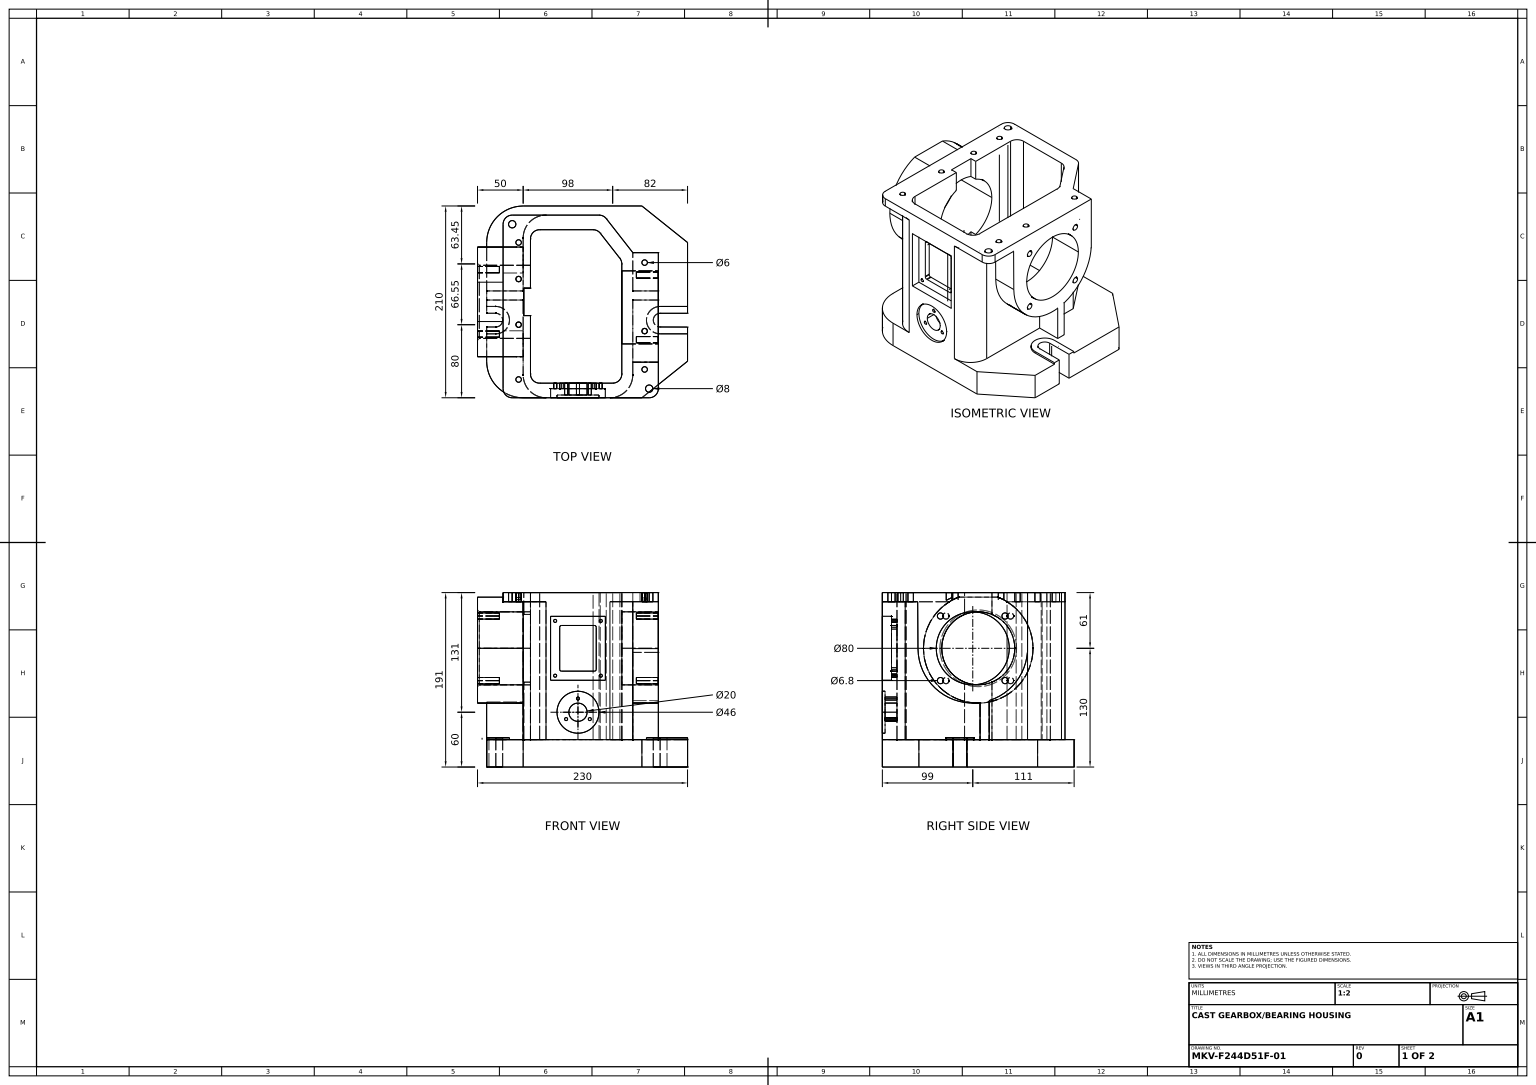
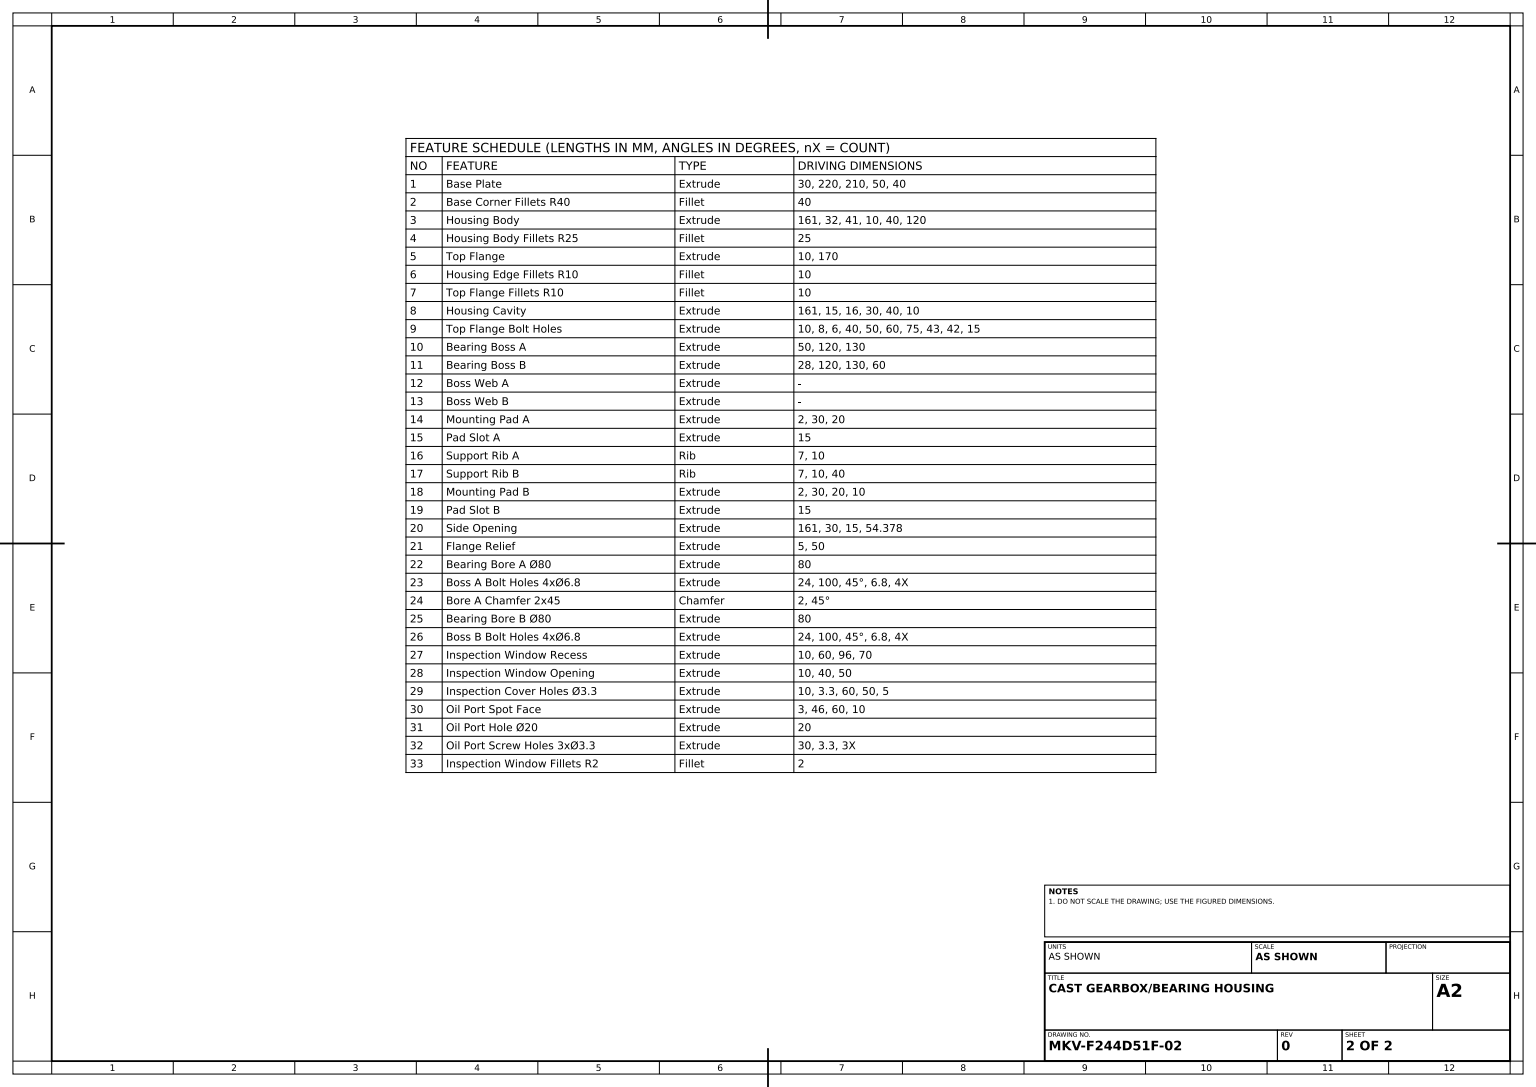
SolidWorks part; units mm, degrees
material "Cast Carbon Steel"
ref_plane "Front Plane" through (0, 0, 0) normal (0, 0, 1) x (1, 0, 0)
ref_plane "Top Plane" through (0, 0, 0) normal (0, 1, 0) x (1, 0, 0)
ref_plane "Right Plane" through (0, 0, 0) normal (1, 0, 0) x (0, 0, -1)
sketch "Base Plate Sketch" plane through (0, 0, 0) normal (0, 1, 0) x (1, 0, 0)
  line L0 (60, 105) -> (110, 65)
  line L1 (-110, -105) -> (60, -105)
  line L2 (-110, -105) -> (-110, 105)
  line L3 (-110, 105) -> (60, 105)
  line L4 (110, -65) -> (110, 65)
  line L5 (-110, -105) -> (110, 105) construction
  line L6 (-110, 105) -> (110, -105) construction
  line L7 (60, -105) -> (110, -65)
  point P0 (0, 0)
  dimension "D1" = 220
  dimension "D2" = 210
  dimension "D3" = 50
  dimension "D4" = 40
  dimension "D5" = 50
  dimension "D6" = 40
extrude "Base Plate" add sketch "Base Plate Sketch" along normal blind 30
fillet "Base Corner Fillets R40" radius 40 2 edges at (-110, 15, -105) (-110, 15, 105)
sketch "Housing Body Sketch" plane through (0, 30, 0) normal (0, 1, 0) x (1, 0, 0)
  line L0 (-70, -105) -> (60, -105) construction
  line L1 (-70, 95) -> (18, 95)
  line L2 (-70, 95) -> (-70, -105)
  line L3 (-70, -105) -> (50, -105)
  line L4 (50, 54) -> (50, -105)
  line L5 (18, 95) -> (50, 54)
  line L6 (60, 105) -> (-70, 105) construction
  line L7 (-110, 65) -> (-110, -65) construction
  dimension "D1" = 32
  dimension "D2" = 41
  dimension "D3" = 10
  dimension "D4" = 40
  dimension "D5" = 120
extrude "Housing Body" add sketch "Housing Body Sketch" along normal blind 161
fillet "Housing Body Fillets R25" radius 25 3 edges at (-70, 110.5, -95) (-70, 110.5, 105) (50, 110.5, 105)
sketch "Top Flange Sketch" plane through (0, 191, 0) normal (0, 1, 0) x (1, 0, 0)
  line L0 (18, 95) -> (-92, 95)
  line L1 (-92, 95) -> (-92, -105)
  line L2 (-92, -105) -> (78, -105)
  line L3 (78, -105) -> (78, 54)
  line L4 (78, 54) -> (50, 54)
  line L5 (50, 54) -> (18, 95)
  line L6 (-70, 70) -> (-70, -80) construction
  dimension "D1" = 170
  dimension "D2" = 148
extrude "Top Flange" add sketch "Top Flange Sketch" against normal blind 10
fillet "Housing Edge Fillets R10" radius 10 1 edges at (18, 110.5, -95)
fillet "Top Flange Fillets R10" radius 10 3 edges at (78, 186, 105) (-92, 186, 105) (-92, 186, -95)
sketch "Housing Cavity Sketch" plane through (0, 191, 0) normal (0, 1, 0) x (1, 0, 0)
  line L2 (38.1753, 44.7709) -> (9.178, 81.9236)
  line L3 (35.8832, 47.7077) -> (14.4627, 75.1527)
  line L5 (13.1196, 79) -> (-82, 79)
  line L6 (6.5795, 79) -> (-52, 79)
  line L8 (-62, 85) -> (-62, -95)
  line L9 (-62, 69) -> (-62, -79)
  line L11 (-82, -89) -> (68, -89)
  line L12 (-52, -89) -> (28, -89)
  line L14 (38, -95) -> (38, 54)
  line L15 (38, -79) -> (38, 41.555)
  arc A0 (6.5795, 79) -> (14.4627, 75.1527) centre (6.5795, 69) cw
  arc A1 (35.8832, 47.7077) -> (38, 41.555) centre (28, 41.555) cw
  arc A2 (28, -89) -> (38, -79) centre (28, -79) ccw
  arc A3 (-52, -89) -> (-62, -79) centre (-52, -79) cw
  arc A4 (-62, 69) -> (-52, 79) centre (-52, 69) cw
  dimension "D6" = 10
  dimension "D1" = 15
  dimension "D2" = 16
  dimension "D3" = 30
  dimension "D4" = 16
  dimension "D5" = 40
extrude "Housing Cavity" cut sketch "Housing Cavity Sketch" against normal blind 161
sketch "Top Flange Bolt Holes Sketch" plane through (0, 191, 0) normal (0, 1, 0) x (1, 0, 0)
  line L0 (0, 0) -> (-14.5243, 0) construction
  line L4 (78, -95) -> (78, 54) construction
  circle A0 centre (-82, 85) radius 4
  circle A1 centre (68, -95) radius 4
  circle A2 centre (-75, 65) radius 3
  circle A3 centre (-75, 25) radius 3
  circle A4 centre (-75, -25) radius 3
  circle A5 centre (-75, -85) radius 3
  circle A6 centre (63, 43) radius 3
  circle A7 centre (63, -32) radius 3
  circle A8 centre (63, -74) radius 3
  dimension "D1" = 8
  dimension "D2" = 6
  dimension "D3" = 40
  dimension "D4" = 50
  dimension "D5" = 60
  dimension "D6" = 75
  dimension "D7" = 43
  dimension "D8" = 75
  dimension "D9" = 42
  dimension "D10" = 15
extrude "Top Flange Bolt Holes" cut sketch "Top Flange Bolt Holes Sketch" against normal blind 10
sketch "Bearing Boss A Sketch" plane through (-70, 0, 0) normal (-1, 0, 0) x (0, 0, 1)
  circle A0 centre (0, 130) radius 60
  dimension "D1" = 120
  dimension "D2" = 130
extrude "Bearing Boss A" add sketch "Bearing Boss A Sketch" along normal blind 50
sketch "Bearing Boss B Sketch" plane through (50, 0, 0) normal (1, 0, 0) x (0, 0, -1)
  line L0 (54, 181) -> (54, 30) construction
  circle A0 centre (-6, 130) radius 60
  dimension "D1" = 120
  dimension "D2" = 130
  dimension "D3" = 60
extrude "Bearing Boss B" add sketch "Bearing Boss B Sketch" along normal blind 28
sketch "Boss Web A Sketch" plane through (0, 0, -54) normal (0, 0, -1) x (-1, 0, 0)
  line L0 (-78, 181) -> (-78, 70) construction
  line L1 (-50, 181) -> (-78, 181)
  line L2 (-50, 181) -> (-50, 125.5)
  line L3 (-50, 125.5) -> (-78, 125.5)
  line L4 (-78, 181) -> (-78, 125.5)
extrude "Boss Web A" add sketch "Boss Web A Sketch" against normal up to next
sketch "Boss Web B Sketch" plane through (78, 0, 0) normal (1, 0, 0) x (0, 0, -1)
  line L0 (-65.9989, 129.6442) -> (-66.3035, 181)
  line L1 (-95, 181) -> (-37.607, 181) construction
  line L2 (-66.3035, 181) -> (-37.607, 181)
  arc A0 (-37.607, 181) -> (53.831, 125.5) centre (-6, 130) ccw construction
  arc A1 (-37.607, 181) -> (53.831, 125.5) centre (-6, 130) ccw construction
  arc A2 (-65.9989, 129.6442) -> (-37.607, 181) centre (-6, 130) cw
extrude "Boss Web B" add sketch "Boss Web B Sketch" against normal up to next
sketch "Mounting Pad A Sketch" plane through (0, 30, 0) normal (0, 1, 0) x (1, 0, 0)
  line L0 (110, -65) -> (110, 65) construction
  line L1 (80, -5) -> (110, -5)
  line L2 (110, -5) -> (110, -35)
  line L3 (110, -35) -> (80, -35)
  arc A0 (80, -5) -> (80, -35) centre (80, -20) ccw
  dimension "D1" = 30
  dimension "D2" = 20
  dimension "D3" = 30
extrude "Mounting Pad A" add sketch "Mounting Pad A Sketch" along normal blind 2
sketch "Pad Slot A Sketch" plane through (0, 32, 0) normal (0, 1, 0) x (1, 0, 0)
  line L0 (80, -12.5) -> (110, -12.5)
  line L1 (110, -35) -> (110, -5) construction
  line L2 (110, -12.5) -> (110, -27.5962)
  line L3 (110, -27.5962) -> (79.976, -27.5)
  arc A0 (80, -12.5) -> (79.976, -27.5) centre (80, -20) ccw
  dimension "D1" = 15
  dimension "D2" = 0.024
extrude "Pad Slot A" cut sketch "Pad Slot A Sketch" against normal through all
ref_plane "Plane2" through (0, 0, -7) normal (0, 0, 1) x (1, 0, 0)
sketch "Support Rib A Sketch" plane through (0, 0, -7) normal (0, 0, 1) x (1, 0, 0)
  line L0 (78, 70) -> (78, 30)
  line L1 (110, 30) -> (60, 30) construction
rib "Support Rib A" sketch "Support Rib A Sketch" sketch "Support Rib A Sketch" thickness 10 extrusion direction parallel to sketch draft on no parameters "D1"=10
sketch "Support Rib B Sketch" plane through (0, 0, -7) normal (0, 0, 1) x (1, 0, 0)
  line L0 (-110, 70) -> (-110, 30)
  line L1 (-120, 70) -> (-70, 70) construction
  line L2 (-70, 30) -> (-110, 30) construction
  line L3 (-70, 30) -> (-70, 181) construction
  dimension "D1" = 40
rib "Support Rib B" sketch "Support Rib B Sketch" sketch "Support Rib B Sketch" thickness 10 extrusion direction parallel to sketch draft on no parameters "D1"=10
sketch "Mounting Pad B Sketch" plane through (0, 30, 0) normal (0, 1, 0) x (1, 0, 0)
  line L0 (-110, 65) -> (-110, 12) construction
  line L1 (-100, -5) -> (-110, -5)
  line L2 (-110, -5) -> (-110, -35)
  line L3 (-110, -35) -> (-100, -35)
  arc A0 (-100, -35) -> (-100, -5) centre (-100, -20) ccw
  dimension "D1" = 30
  dimension "D2" = 20
  dimension "D3" = 10
extrude "Mounting Pad B" add sketch "Mounting Pad B Sketch" along normal blind 2
sketch "Pad Slot B Sketch" plane through (0, 32, 0) normal (0, 1, 0) x (1, 0, 0)
  line L0 (-100, -12.5) -> (-110, -12.5)
  line L1 (-110, -5) -> (-110, -35) construction
  line L2 (-110, -12.5) -> (-110, -27.5)
  line L3 (-110, -27.5) -> (-100, -27.5)
  arc A0 (-100, -27.5) -> (-100, -12.5) centre (-100, -20) ccw
  dimension "D1" = 15
extrude "Pad Slot B" cut sketch "Pad Slot B Sketch" against normal through all
sketch "Side Opening Sketch" plane through (0, 191, 0) normal (0, 1, 0) x (1, 0, 0)
  line L0 (0, 0) -> (-14.6419, 0) construction
  line L1 (-69.378, 15) -> (-54.378, 15)
  line L2 (-69.378, 15) -> (-69.378, -15)
  line L3 (-69.378, -15) -> (-54.378, -15)
  line L4 (-54.378, 15) -> (-54.378, -15)
  dimension "D1" = 30
  dimension "D2" = 15
  dimension "D3" = 54.378
extrude "Side Opening" cut sketch "Side Opening Sketch" against normal blind 161
sketch "Flange Relief Sketch" plane through (0, 191, 0) normal (0, 1, 0) x (1, 0, 0)
  line L0 (-92, 31.607) -> (-92, -31.607) construction
  line L1 (-92, 25) -> (-120, 25)
  line L2 (-92, 25) -> (-92, -25)
  line L3 (-92, -25) -> (-120, -25)
  line L4 (-120, 25) -> (-120, -25)
  line L5 (-120, 60) -> (-120, -60) construction
  line L6 (0, 0) -> (-14.0575, 0) construction
  dimension "D1" = 50
extrude "Flange Relief" cut sketch "Flange Relief Sketch" against normal blind 5
sketch "Bearing Bore A Sketch" plane through (-120, 0, 0) normal (-1, 0, 0) x (0, 0, 1)
  circle A0 centre (0, 130) radius 40
  dimension "D1" = 80
extrude "Bearing Bore A Ø80" cut sketch "Bearing Bore A Sketch" against normal up to next
sketch "Boss A Bolt Holes Sketch" plane through (-120, 0, 0) normal (-1, 0, 0) x (0, 0, 1)
  line L0 (0, 130) -> (38.4228, 91.5772) construction
  circle A0 centre (0, 130) radius 50 construction
  circle A1 centre (35.3553, 94.6447) radius 3.4
  circle A2 centre (-35.3553, 94.6447) radius 3.4
  circle A3 centre (-35.3553, 165.3553) radius 3.4
  circle A4 centre (35.3553, 165.3553) radius 3.4
  dimension "D1" = 100
  dimension "D3" = 6.8
  dimension "D2" = 45
  dimension "D4" = 4
extrude "Boss A Bolt Holes 4xØ6.8" cut sketch "Boss A Bolt Holes Sketch" against normal blind 24
chamfer "Bore A Chamfer 2x45" distance 2 angle 45 1 edges at (-120, 130, 40)
sketch "Bearing Bore B Sketch" plane through (78, 0, 0) normal (1, 0, 0) x (0, 0, -1)
  circle A0 centre (-6, 130) radius 40
  dimension "D1" = 80
extrude "Bearing Bore B Ø80" cut sketch "Bearing Bore B Sketch" against normal up to next
sketch "Boss B Bolt Holes Sketch" plane through (78, 0, 0) normal (1, 0, 0) x (0, 0, -1)
  line L0 (-6, 130) -> (33.9986, 90.0014) construction
  circle A0 centre (-6, 130) radius 50 construction
  circle A1 centre (29.3553, 94.6447) radius 3.4
  circle A2 centre (-41.3553, 94.6447) radius 3.4
  circle A3 centre (-41.3553, 165.3553) radius 3.4
  circle A4 centre (29.3553, 165.3553) radius 3.4
  dimension "D1" = 100
  dimension "D3" = 6.8
  dimension "D2" = 45
  dimension "D4" = 4
extrude "Boss B Bolt Holes 4xØ6.8" cut sketch "Boss B Bolt Holes Sketch" against normal blind 24
sketch "Inspection Window Recess Sketch" plane through (0, 0, 105) normal (0, 0, 1) x (1, 0, 0)
  line L0 (-82, 191) -> (68, 191) construction
  line L1 (-40, 165) -> (20, 165)
  line L2 (-40, 165) -> (-40, 95)
  line L3 (-40, 95) -> (20, 95)
  line L4 (20, 165) -> (20, 95)
  point P4 (-10, 95)
  dimension "D1" = 60
  dimension "D2" = 10
  dimension "D3" = 96
  dimension "D4" = 70
extrude "Inspection Window Recess" cut sketch "Inspection Window Recess Sketch" against normal blind 10
sketch "Inspection Window Opening Sketch" plane through (0, 0, 95) normal (0, 0, 1) x (1, 0, 0)
  line L0 (-40, 95) -> (20, 95) construction
  line L1 (-30, 105) -> (10, 105)
  line L2 (-30, 105) -> (-30, 155)
  line L3 (-30, 155) -> (10, 155)
  line L4 (10, 105) -> (10, 155)
  line L5 (-30, 105) -> (10, 155) construction
  line L6 (-30, 155) -> (10, 105) construction
  point P0 (-10, 130)
  dimension "D1" = 40
  dimension "D2" = 50
  dimension "D3" = 10
  dimension "D4" = 10
extrude "Inspection Window Opening" cut sketch "Inspection Window Opening Sketch" against normal blind 10
sketch "Inspection Cover Holes Sketch" plane through (0, 0, 95) normal (0, 0, 1) x (1, 0, 0)
  line L0 (-10, 105) -> (-10, 116.7621) construction
  line L1 (-30, 105) -> (10, 105) construction
  line L2 (20, 165) -> (-40, 165) construction
  circle A0 centre (-35, 160) radius 1.65
  circle A1 centre (15, 160) radius 1.65
  circle A2 centre (-35, 100) radius 1.65
  circle A3 centre (15, 100) radius 1.65
  dimension "D1" = 3.3
  dimension "D2" = 60
  dimension "D3" = 50
  dimension "D4" = 5
extrude "Inspection Cover Holes Ø3.3" cut sketch "Inspection Cover Holes Sketch" against normal blind 10
sketch "Oil Port Spot Face Sketch" plane through (0, 0, 105) normal (0, 0, 1) x (1, 0, 0)
  line L0 (-70, 0) -> (60, 0) construction
  circle A0 centre (-10, 60) radius 23
  dimension "D1" = 46
  dimension "D2" = 60
  dimension "D3" = 10
extrude "Oil Port Spot Face" cut sketch "Oil Port Spot Face Sketch" against normal blind 3
sketch "Oil Port Hole Sketch" plane through (0, 0, 102) normal (0, 0, 1) x (1, 0, 0)
  circle A0 centre (-10, 60) radius 10
  dimension "D1" = 20
extrude "Oil Port Hole Ø20" cut sketch "Oil Port Hole Sketch" against normal up to next
sketch "Oil Port Screw Holes Sketch" plane through (0, 0, 102) normal (0, 0, 1) x (1, 0, 0)
  circle A0 centre (-10, 60) radius 15 construction
  circle A1 centre (-10, 75) radius 1.65
  circle A2 centre (2.9904, 52.5) radius 1.65
  circle A3 centre (-22.9904, 52.5) radius 1.65
  dimension "D1" = 30
  dimension "D2" = 3.3
  dimension "D3" = 3
extrude "Oil Port Screw Holes 3xØ3.3" cut sketch "Oil Port Screw Holes Sketch" against normal up to next
fillet "Inspection Window Fillets R2" radius 2 4 edges at (-30, 105, 92) (-30, 155, 92) (10, 155, 92) (10, 105, 92)
